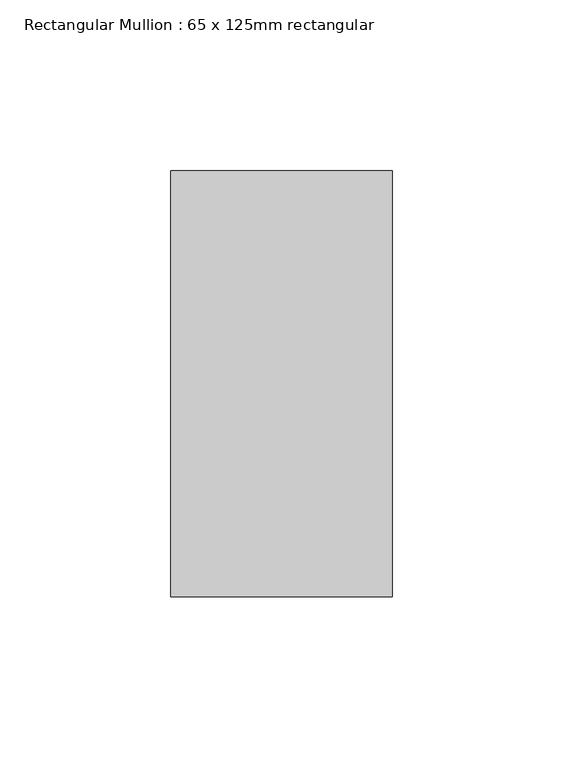
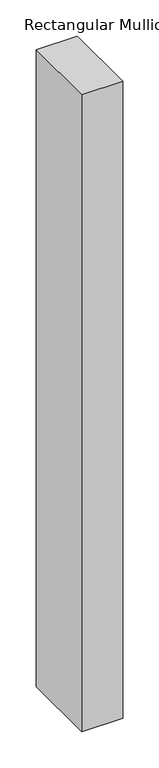
"""IFC4 building model written with IfcOpenShell, lengths in millimetres: member geometry, Rectangular Mullion : 65 x 125mm rectangular."""

from ifc_helpers import new_model, si_unit, frame, origin, place, context, project, spatial, polyline, outline, extrude, source, transform, mapped, element, save


def rectangular_mullion_65_x_125mm_rectangular_ca84e85e(model_context):
    return source(origin(), model_context, "Body", "SweptSolid", [
        extrude(outline(polyline([(32.5, 62.5), (32.5, -62.5), (-32.5, -62.5), (-32.5, 62.5), (32.5, 62.5)])), frame((0.0, 0.0, -1070.0), z_axis=(0.0, 0.0, 1.0), x_axis=(1.0, 0.0, 0.0)), (0.0, 0.0, 1.0), 1070.0),
    ])


if __name__ == "__main__":
    model = new_model("IFC4")
    model_context = context("Model", 3, world=origin())
    ifc_project = project(units=[si_unit("LENGTHUNIT", "METRE", prefix="MILLI")], contexts=[model_context])
    site = spatial("IfcSite", under=ifc_project)
    building = spatial("IfcBuilding", under=site)
    placement = place(None, origin())
    rectangular_mullion_65_x_125mm_rectangular_shape = rectangular_mullion_65_x_125mm_rectangular_ca84e85e(model_context)
    element("IfcMember", 1, ObjectType="Rectangular Mullion : 65 x 125mm rectangular", at=placement, inside=building, context=model_context, shape_type="MappedRepresentation", body=[
        mapped(rectangular_mullion_65_x_125mm_rectangular_shape, transform((0.0, 0.0, 0.0), x_axis=(1.0, 0.0, 0.0), y_axis=(0.0, 1.0, 0.0), z_axis=(0.0, 0.0, 1.0))),
    ])
    save(model, "model.ifc")

# Revit data of these elements
# Type "Rectangular Mullion : 65 x 125mm rectangular"
#   built-in parameter 1007304 = 0.410105 (stored number, unit not read)
#   built-in parameter 1007301 = 0.106627 (stored number, unit not read)
#   built-in parameter 1007300 = 0.106627 (stored number, unit not read)
# Element 1 (IfcMember, "Rectangular Mullion : 65 x 125mm rectangular")
#   Materials on its faces: "Aluminum"
# Materials
#   "Aluminum": class "Metal", colour RGB 244 245 246, transparency 0, Description = "Aluminum 6061", Cost = 0
